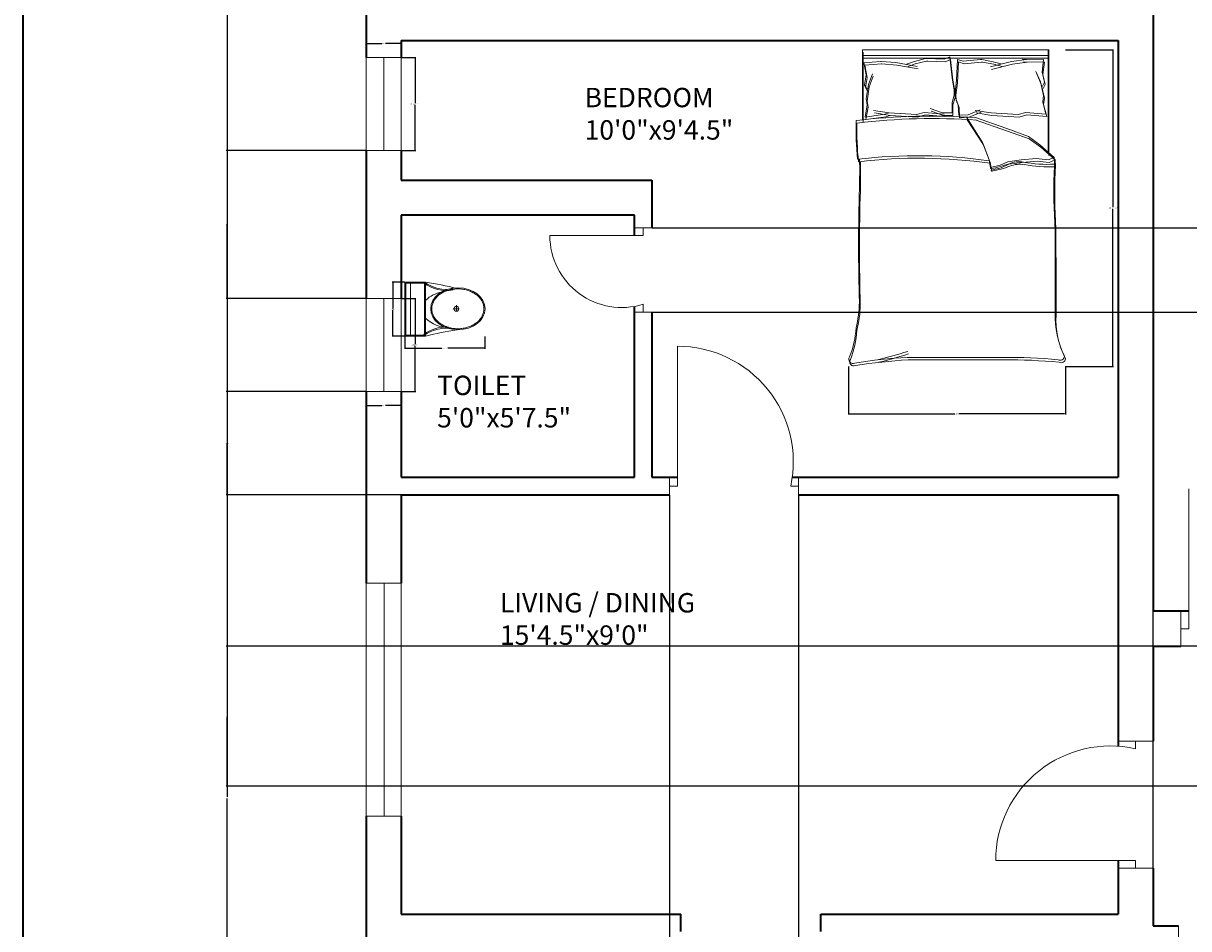
# Model space of a CAD drawing. Units: inches. Extents: x 2527 to 3140, y 1564 to 2435.
# Tile 2 of 4: x 2527 to 2827, y 1993 to 2227. Entities that reach past the tile are written whole.
import ezdxf

# ---------------------------------------------------------------- set-up
doc = ezdxf.new("R2010")
doc.units = ezdxf.units.IN
for name, color, linetype, lineweight in [('A-ANNO-DIMS', 2, 'Continuous', 18), ('A-ANNO-TTLB', 7, 'Continuous', 35), ('A-AREA-IDEN', 7, 'Continuous', 18), ('A-DOOR', 191, 'Continuous', 18), ('A-FLOR-FIXT', 7, 'Continuous', 18), ('A-FURN', 8, 'Continuous', 13), ('A-GLAZ', 131, 'Continuous', 18), ('A-WALL', 7, 'Continuous', 35)]:
    doc.layers.add(name, color=color, linetype=linetype, lineweight=lineweight)
doc.styles.get("Standard").update_dxf_attribs({"font": 'arial.ttf'})
doc.dimstyles.get("Standard").update_dxf_attribs({"dimtxt": 0.18, "dimasz": 0.18, "dimexe": 0.18, "dimexo": 0.0625, "dimgap": 0.09, "dimtad": 0, "dimtih": 1, "dimtoh": 1, "dimdec": 4, "dimzin": 0, "dimdsep": 46, "dimtxsty": 'Standard', "dimcen": 0.09, "dimadec": 0, "dimazin": 0, "dimtfac": 1, "dimtdec": 4, "dimtofl": 0, "dimtmove": 0, "dimatfit": 3, "dimfxl": 1, "dimtolj": 1, "dimtzin": 0, "dimarcsym": 0})

# ---------------------------------------------------------------- blocks, each defined once
blk = doc.blocks.new('A$C31115884')
for p, q in [((283, 498), (223, 498)), ((258, 466), (258, 523)), ((0, 200), (0, 0)), ((520, 200), (0, 200)), ((10, 190), (10, 10)), ((510, 190), (10, 190)), ((510, 10), (510, 190)), ((520, 0), (520, 200)), ((510, 54), (0, 54)), ((10, 10), (510, 10)), ((0, 0), (520, 0))]:
    blk.add_line(p, q)
blk.add_circle((256, 496), 23.6)
for centre, radius, start, end in [((2778, -205), 2807, 165.4549, 171.7133), ((-295, 403), 365, 324.2091, 9.3499), ((-295, 403), 375, 324.2091, 9.3499), ((806, 403), 365, 170.6501, 215.7909), ((3237, 905), 2807, 188.2867, 194.5451), ((384, 406), 293, 190.2774, 224.1564), ((139, 406), 293, 315.8436, 2.6563), ((806, 403), 375, 179.2036, 215.7909)]:
    blk.add_arc(centre, radius, start, end)
blk.add_ellipse((256, 510), major_axis=(0, -261), ratio=0.772727)
blk.add_open_spline([(256, 259), (263, 259), (270, 260), (288, 262), (299, 265), (320, 273), (330, 278), (350, 291), (360, 299), (378, 316), (386, 326), (402, 347), (409, 358), (421, 383), (427, 395), (436, 422), (440, 436), (445, 465), (447, 480), (448, 509), (448, 524), (445, 553), (443, 568), (436, 596), (432, 610), (422, 636), (416, 649), (402, 672), (395, 683), (379, 703), (370, 712), (351, 728), (341, 735), (321, 746), (310, 751), (289, 757), (278, 759), (256, 761), (245, 761), (223, 757), (212, 754), (191, 746), (181, 741), (161, 728), (151, 720), (133, 703), (125, 693), (110, 672), (103, 660), (90, 636), (85, 623), (76, 596), (72, 582), (67, 553), (66, 538), (64, 509), (65, 494), (68, 465), (70, 450), (77, 422), (81, 408), (91, 382), (97, 370), (111, 346), (118, 335), (135, 316), (144, 307), (162, 291), (172, 284), (193, 273), (203, 269), (225, 262), (236, 260), (250, 259), (253, 259), (256, 259)], degree=3, knots=[0, 0, 0, 0, 0.110105, 0.110105, 0.285049, 0.285049, 0.459994, 0.459994, 0.634938, 0.634938, 0.809882, 0.809882, 0.984827, 0.984827, 1.159771, 1.159771, 1.334715, 1.334715, 1.50966, 1.50966, 1.684604, 1.684604, 1.859549, 1.859549, 2.034493, 2.034493, 2.209437, 2.209437, 2.384382, 2.384382, 2.559326, 2.559326, 2.73427, 2.73427, 2.909215, 2.909215, 3.084159, 3.084159, 3.259103, 3.259103, 3.434048, 3.434048, 3.608992, 3.608992, 3.783936, 3.783936, 3.958881, 3.958881, 4.133825, 4.133825, 4.30877, 4.30877, 4.483714, 4.483714, 4.658658, 4.658658, 4.833603, 4.833603, 5.008547, 5.008547, 5.183491, 5.183491, 5.358436, 5.358436, 5.53338, 5.53338, 5.708324, 5.708324, 5.883269, 5.883269, 6.058213, 6.058213, 6.233158, 6.233158, 6.283185, 6.283185, 6.283185, 6.283185])
blk = doc.blocks.new('BED-DOUBLE')
for p, q in [((3.48, 63.33), (3.48, 81.44)), ((3.48, 63.33), (3.48, 81.44)), ((3.48, 81.44), (51.49, 81.44)), ((51.27, 81.44), (51.27, 54.83)), ((51.27, 81.44), (51.27, 54.83)), ((51.49, 81.44), (51.49, 80.8)), ((3.48, 79.91), (51.27, 79.91)), ((3.48, 79.91), (51.27, 79.91)), ((3.7, 62.69), (3.7, 80.8)), ((3.7, 62.69), (3.7, 80.8)), ((3.7, 79.27), (51.49, 79.27)), ((3.7, 79.27), (51.49, 79.27)), ((3.89, 78.13), (4.47, 74.95)), ((3.9, 78.1), (8.18, 78.43)), ((3.9, 78.1), (8.18, 78.43)), ((3.9, 78.13), (4.47, 74.95)), ((8.18, 78.43), (8.29, 78.42)), ((8.18, 78.43), (8.29, 78.42)), ((8.29, 78.42), (12.11, 78.13)), ((8.29, 78.42), (12.11, 78.13)), ((12.11, 78.13), (17.6, 77.11)), ((12.11, 78.13), (17.6, 77.11)), ((14.86, 77.69), (16.88, 78.42)), ((14.86, 77.69), (16.88, 78.42)), ((16.88, 78.42), (19.77, 79.14)), ((16.88, 78.42), (19.77, 79.14)), ((17.11, 77.78), (20, 78.5)), ((17.11, 77.78), (20, 78.5)), ((19.77, 79.14), (20.09, 79.14)), ((19.77, 79.14), (20.09, 79.14)), ((20, 78.5), (20.32, 78.5)), ((20, 78.5), (20.32, 78.5)), ((20.09, 79.14), (24.54, 78.99)), ((20.09, 79.14), (24.54, 78.99)), ((20.32, 78.5), (24.77, 78.35)), ((20.32, 78.5), (24.77, 78.35)), ((24.54, 78.99), (25.98, 79.57)), ((24.54, 78.99), (25.98, 79.57)), ((24.77, 78.35), (26.21, 78.93)), ((24.77, 78.35), (26.21, 78.93)), ((25.98, 79.57), (26.56, 74.22)), ((25.98, 79.57), (26.56, 74.22)), ((26.21, 78.93), (26.79, 73.58)), ((26.21, 78.93), (26.79, 73.58)), ((27.98, 78.95), (27.73, 73.58)), ((27.98, 78.95), (27.73, 73.58)), ((28.21, 78.31), (27.96, 72.94)), ((28.21, 78.31), (27.96, 72.94)), ((29.46, 78.46), (27.98, 78.95)), ((29.46, 78.46), (27.98, 78.95)), ((29.68, 77.82), (28.21, 78.31)), ((29.68, 77.82), (28.21, 78.31)), ((33.88, 78.89), (29.46, 78.46)), ((33.88, 78.89), (29.46, 78.46)), ((34.11, 78.25), (29.68, 77.82)), ((34.11, 78.25), (29.68, 77.82)), ((34.21, 78.91), (33.88, 78.89)), ((34.2, 78.91), (33.88, 78.89)), ((34.43, 78.27), (34.11, 78.25)), ((34.43, 78.27), (34.11, 78.25)), ((37.14, 78.36), (34.2, 78.91)), ((37.14, 78.36), (34.21, 78.91)), ((37.36, 77.73), (34.43, 78.27)), ((37.36, 77.73), (34.43, 78.27)), ((41.91, 78.37), (36.5, 77.02)), ((41.91, 78.37), (36.5, 77.02)), ((39.2, 77.77), (37.14, 78.36)), ((39.2, 77.77), (37.14, 78.36)), ((45.71, 78.9), (41.91, 78.37)), ((45.71, 78.9), (41.91, 78.37)), ((45.94, 78.26), (42.14, 77.73)), ((45.94, 78.26), (42.14, 77.73)), ((50.11, 78.89), (44.71, 78.98)), ((44.71, 78.98), (45.71, 78.9)), ((50.11, 78.89), (44.71, 78.98)), ((44.71, 78.98), (45.71, 78.9)), ((50.34, 78.25), (44.94, 78.34)), ((44.94, 78.34), (45.94, 78.26)), ((50.34, 78.25), (44.94, 78.34)), ((44.94, 78.34), (45.94, 78.26)), ((50.11, 78.89), (49.73, 75.68)), ((50.11, 78.89), (49.73, 75.68)), ((50.34, 78.25), (49.96, 75.04)), ((50.34, 78.25), (49.96, 75.04)), ((51.49, 80.8), (51.49, 54.19)), ((51.49, 80.8), (51.49, 54.19)), ((4.12, 77.49), (4.7, 74.31)), ((4.12, 77.49), (4.7, 74.31)), ((4.13, 77.47), (8.41, 77.79)), ((4.13, 77.47), (8.41, 77.79)), ((5.05, 72.49), (6.06, 75.24)), ((5.05, 72.49), (6.06, 75.24)), ((8.41, 77.79), (8.51, 77.78)), ((8.41, 77.79), (8.51, 77.78)), ((8.51, 77.78), (12.34, 77.49)), ((8.51, 77.78), (12.34, 77.49)), ((12.34, 77.49), (17.83, 76.48)), ((12.34, 77.49), (17.83, 76.48)), ((15.08, 77.05), (17.11, 77.78)), ((15.08, 77.05), (17.11, 77.78)), ((42.14, 77.73), (36.72, 76.38)), ((42.14, 77.73), (36.72, 76.38)), ((39.43, 77.13), (37.36, 77.73)), ((39.43, 77.13), (37.36, 77.73)), ((49.31, 73.19), (48.13, 75.86)), ((49.31, 73.19), (48.13, 75.86)), ((49.54, 72.55), (48.36, 75.23)), ((49.54, 72.55), (48.36, 75.23)), ((49.73, 75.68), (50.33, 73.1)), ((49.73, 75.68), (50.33, 73.1)), ((49.96, 75.04), (50.56, 72.47)), ((49.96, 75.04), (50.56, 72.47)), ((4.47, 74.95), (4.04, 72.34)), ((4.47, 74.95), (4.04, 72.34)), ((4.04, 72.34), (4.62, 71.33)), ((4.04, 72.34), (4.62, 71.33)), ((4.7, 74.31), (4.27, 71.7)), ((4.7, 74.31), (4.27, 71.7)), ((4.47, 68.87), (5.05, 72.49)), ((4.47, 68.87), (5.05, 72.49)), ((5.28, 71.85), (6.29, 74.6)), ((5.28, 71.85), (6.29, 74.6)), ((26.56, 74.22), (27.14, 71.04)), ((26.56, 74.22), (27.14, 71.04)), ((26.79, 73.58), (27.37, 70.4)), ((26.79, 73.58), (27.37, 70.4)), ((27.73, 73.58), (27.36, 70.36)), ((27.73, 73.58), (27.36, 70.36)), ((27.96, 72.94), (27.58, 69.73)), ((27.96, 72.94), (27.58, 69.73)), ((50.11, 69.61), (49.31, 73.19)), ((50.11, 69.61), (49.31, 73.19)), ((50.34, 68.97), (49.54, 72.55)), ((50.34, 68.97), (49.54, 72.55)), ((50.33, 73.1), (49.81, 72.06)), ((50.33, 73.1), (49.82, 72.06)), ((50.56, 72.47), (50.04, 71.42)), ((50.56, 72.47), (50.04, 71.42)), ((4.27, 71.7), (4.85, 70.69)), ((4.27, 71.7), (4.85, 70.69)), ((4.7, 68.23), (5.28, 71.85)), ((4.7, 68.23), (5.28, 71.85)), ((27.14, 69.74), (26.56, 67.86)), ((27.14, 69.74), (26.56, 67.86)), ((27.37, 69.1), (26.79, 67.22)), ((27.37, 69.1), (26.79, 67.22)), ((27.14, 71.04), (27.14, 69.74)), ((27.14, 71.04), (27.14, 69.74)), ((27.36, 70.36), (27.44, 69.07)), ((27.36, 70.36), (27.44, 69.07)), ((27.37, 70.4), (27.37, 69.1)), ((27.37, 70.4), (27.37, 69.1)), ((27.44, 69.07), (28.13, 67.23)), ((27.44, 69.07), (28.13, 67.23)), ((27.58, 69.73), (27.66, 68.43)), ((27.58, 69.73), (27.66, 68.43)), ((49.92, 68.01), (50.11, 69.61)), ((49.92, 68.01), (50.11, 69.61)), ((4.18, 64.1), (4.76, 67.28)), ((4.18, 64.1), (4.76, 67.28)), ((4.41, 63.46), (4.99, 66.64)), ((4.41, 63.46), (4.99, 66.64)), ((4.76, 67.28), (4.47, 68.87)), ((4.76, 67.28), (4.47, 68.87)), ((4.99, 66.64), (4.7, 68.23)), ((4.99, 66.64), (4.7, 68.23)), ((24.1, 65.18), (20.96, 66.27)), ((24.1, 65.18), (20.96, 66.27)), ((26.56, 67.86), (26.56, 65.18)), ((26.56, 67.86), (26.56, 65.18)), ((26.79, 67.22), (26.79, 64.54)), ((26.79, 67.22), (26.79, 64.54)), ((27.66, 68.43), (28.36, 66.59)), ((27.66, 68.43), (28.36, 66.59)), ((28.13, 67.23), (28.3, 64.55)), ((28.13, 67.23), (28.3, 64.55)), ((28.36, 66.59), (28.53, 63.91)), ((28.36, 66.59), (28.53, 63.91)), ((50.7, 64.87), (49.92, 68.01)), ((50.7, 64.87), (49.92, 68.01)), ((50.15, 67.37), (50.34, 68.97)), ((50.15, 67.37), (50.34, 68.97)), ((50.93, 64.23), (50.15, 67.37)), ((50.93, 64.23), (50.15, 67.37)), ((9.28, 64.82), (4.18, 64.1)), ((9.28, 64.82), (4.18, 64.1)), ((9.51, 64.19), (4.41, 63.46)), ((9.51, 64.19), (4.41, 63.46)), ((6.38, 65.81), (10.41, 65.15)), ((6.38, 65.81), (10.41, 65.15)), ((6.61, 65.17), (10.64, 64.51)), ((6.61, 65.17), (10.64, 64.51)), ((10.41, 65.15), (9.28, 64.82)), ((10.41, 65.15), (9.28, 64.82)), ((10.64, 64.51), (9.51, 64.19)), ((10.64, 64.51), (9.51, 64.19)), ((10.41, 65.15), (17.42, 64.72)), ((10.41, 65.15), (17.42, 64.72)), ((10.64, 64.51), (17.65, 64.08)), ((10.64, 64.51), (17.65, 64.08)), ((17.42, 64.72), (19.38, 65.27)), ((17.42, 64.72), (19.38, 65.27)), ((17.65, 64.08), (19.61, 64.63)), ((17.65, 64.08), (19.61, 64.63)), ((19.38, 65.27), (24.52, 64.87)), ((19.38, 65.27), (24.52, 64.87)), ((19.61, 64.63), (24.74, 64.23)), ((19.61, 64.63), (24.74, 64.23)), ((24.33, 64.54), (21.19, 65.63)), ((24.33, 64.54), (21.19, 65.63)), ((26.56, 65.18), (24.1, 65.18)), ((26.56, 65.18), (24.1, 65.18)), ((26.79, 64.54), (24.33, 64.54)), ((26.79, 64.54), (24.33, 64.54)), ((28.3, 64.55), (30.75, 64.7)), ((28.3, 64.55), (30.75, 64.7)), ((28.53, 63.91), (30.98, 64.06)), ((28.53, 63.91), (30.98, 64.06)), ((30.26, 64.06), (34.45, 57.57)), ((30.26, 64.06), (34.45, 57.57)), ((30.49, 63.42), (34.68, 56.93)), ((30.49, 63.42), (34.68, 56.93)), ((30.75, 64.7), (33.82, 65.99)), ((30.75, 64.7), (33.82, 65.99)), ((30.98, 64.06), (34.05, 65.35)), ((30.98, 64.06), (34.05, 65.35)), ((40.64, 61.13), (32.31, 64.06)), ((40.64, 61.13), (32.31, 64.06)), ((40.87, 60.49), (32.53, 63.42)), ((40.87, 60.49), (32.54, 63.42)), ((32.56, 65.81), (36.6, 65.15)), ((32.56, 65.81), (36.6, 65.15)), ((32.79, 65.17), (36.83, 64.51)), ((32.79, 65.17), (36.82, 64.51)), ((36.6, 65.15), (43.61, 64.72)), ((36.6, 65.15), (43.61, 64.72)), ((36.82, 64.51), (43.83, 64.08)), ((36.83, 64.51), (43.84, 64.08)), ((43.61, 64.72), (45.57, 65.27)), ((43.61, 64.72), (45.57, 65.27)), ((43.83, 64.08), (45.8, 64.63)), ((43.84, 64.08), (45.8, 64.63)), ((45.57, 65.27), (50.7, 64.87)), ((45.57, 65.27), (50.7, 64.87)), ((45.8, 64.63), (50.93, 64.23)), ((45.8, 64.63), (50.93, 64.23)), ((46.22, 59.11), (40.64, 61.13)), ((46.22, 59.11), (40.64, 61.13)), ((46.45, 58.47), (40.87, 60.49)), ((46.45, 58.47), (40.87, 60.49)), ((34.45, 57.57), (36.15, 53.08)), ((34.45, 57.57), (36.15, 53.08)), ((49.16, 56.95), (46.22, 59.11)), ((49.16, 56.95), (46.22, 59.11)), ((49.39, 56.31), (46.45, 58.47)), ((49.39, 56.31), (46.45, 58.47)), ((34.68, 56.93), (36.38, 52.44)), ((34.68, 56.93), (36.38, 52.44)), ((52.87, 53.7), (49.16, 56.95)), ((52.87, 53.7), (49.16, 56.95)), ((53.1, 53.06), (49.39, 56.31)), ((53.1, 53.06), (49.39, 56.31)), ((36.15, 53.08), (36.46, 51.07)), ((36.15, 53.08), (36.46, 51.07)), ((36.38, 52.44), (36.69, 50.43)), ((36.38, 52.44), (36.69, 50.43)), ((36.46, 51.07), (38.94, 51.68)), ((36.46, 51.07), (38.94, 51.68)), ((36.69, 50.43), (39.17, 51.05)), ((36.69, 50.43), (39.17, 51.05)), ((38.94, 51.68), (40.95, 52.61)), ((38.94, 51.68), (40.95, 52.61)), ((39.17, 51.05), (41.18, 51.97)), ((39.17, 51.05), (41.18, 51.97)), ((40.95, 52.61), (44.36, 53.08)), ((40.95, 52.61), (44.36, 53.08)), ((41.18, 51.97), (44.59, 52.44)), ((41.18, 51.97), (44.59, 52.44)), ((44.36, 53.08), (48.23, 53.39)), ((44.36, 53.08), (48.23, 53.39)), ((44.59, 52.44), (48.46, 52.75)), ((44.59, 52.44), (48.46, 52.75)), ((48.23, 53.39), (51.33, 53.08)), ((48.23, 53.39), (51.33, 53.08)), ((48.46, 52.75), (51.56, 52.44)), ((48.46, 52.75), (51.56, 52.44)), ((51.33, 53.08), (52.87, 53.7)), ((51.33, 53.08), (52.87, 53.7)), ((51.56, 52.44), (53.1, 53.06)), ((51.56, 52.44), (53.1, 53.06)), ((52.95, 51.95), (52.87, 53.7, 3.87)), ((52.95, 51.95), (52.87, 53.7, 3.87)), ((53.18, 51.31), (53.1, 53.06, 3.87)), ((53.18, 51.31), (53.1, 53.06, 3.87)), ((15.06, 2.2), (39.68, 2.2)), ((15.06, 2.2), (39.68, 2.2)), ((15.29, 1.56), (39.91, 1.56)), ((15.29, 1.56), (39.91, 1.56))]:
    blk.add_line(p, q)
for centre, radius, start, end in [((85.16, 61.35), 83.31, 178.7218, 185.604), ((85.16, 61.35), 83.31, 178.7218, 185.604), ((21.36, -100.61), 164.97, 86.0865, 96.7821), ((21.36, -100.61), 164.97, 86.0865, 96.7821), ((21.59, -101.25), 164.97, 86.0865, 96.7821), ((21.59, -101.25), 164.97, 86.0865, 96.7821), ((85.39, 60.71), 83.31, 178.7218, 185.604), ((85.39, 60.71), 83.31, 178.7218, 185.604), ((17.76, -74.87), 129.02, 81.7845, 96.9006), ((17.76, -74.87), 129.02, 81.7845, 96.9006), ((17.98, -75.51), 129.02, 81.7845, 96.9006), ((17.98, -75.51), 129.02, 81.7845, 96.9006), ((-167.31, 50.27), 170.11, 358.4762, 1.0082), ((-167.31, 50.27), 170.11, 358.4762, 1.0082), ((-167.08, 49.63), 170.11, 358.4762, 1.0082), ((-167.08, 49.63), 170.11, 358.4762, 1.0082), ((36.64, 51), 0.185, 160.2464, 271.1377), ((36.64, 51), 0.185, 160.2464, 271.1377), ((31.15, 79.96), 29.65, 280.6617, 289.8806), ((31.15, 79.96), 29.65, 280.6617, 289.8806), ((31.38, 79.32), 29.65, 280.6617, 289.8806), ((31.38, 79.32), 29.65, 280.6617, 289.8806), ((43.74, 46.38), 6.22, 78.6608, 113.7384), ((43.74, 46.38), 6.22, 78.6608, 113.7384), ((43.97, 45.74), 6.22, 78.6608, 113.7384), ((43.97, 45.74), 6.22, 78.6608, 113.7384), ((51.33, 88.1), 36.18, 259.8763, 272.5657), ((51.33, 88.1), 36.18, 259.8763, 272.5657), ((51.56, 87.46), 36.18, 259.8763, 272.5657), ((51.56, 87.46), 36.18, 259.8763, 272.5657), ((182.27, 45.13), 129.5, 176.9791, 183.8365), ((182.27, 45.13), 129.5, 176.9791, 183.8365), ((182.49, 44.49), 129.5, 176.9791, 183.8365), ((182.49, 44.49), 129.5, 176.9791, 183.8365), ((36.87, 50.36), 0.185, 160.2464, 271.1377), ((36.86, 50.36), 0.185, 160.2464, 271.1377), ((484.82, 30.83), 482.31, 178.2277, 181.7185), ((484.82, 30.83), 482.31, 178.2277, 181.7185), ((485.05, 30.19), 482.31, 178.2277, 181.7185), ((485.05, 30.19), 482.31, 178.2277, 181.7185), ((-4508.74, 13.62), 4561.86, 0.00217, 0.28689), ((-4508.74, 13.62), 4561.86, 0.00217, 0.28689), ((-4508.51, 12.98), 4561.86, 0.00217, 0.28689), ((-4508.51, 12.98), 4561.86, 0.00217, 0.28689), ((-26.9, 16.93), 29.63, 346.0648, 358.9113), ((-26.9, 16.93), 29.63, 346.0648, 358.9113), ((-26.67, 16.29), 29.63, 346.0648, 358.9113), ((-26.67, 16.29), 29.63, 346.0648, 358.9113), ((76.16, 12.78), 23.07, 177.4714, 206.4681), ((76.16, 12.78), 23.07, 177.4714, 206.4681), ((76.39, 12.14), 23.07, 177.4714, 206.4681), ((76.39, 12.14), 23.07, 177.4714, 206.4681), ((-21.66, 11.17), 23.56, 337.9751, 356.652), ((-21.66, 11.17), 23.56, 337.9751, 356.652), ((-21.43, 10.53), 23.56, 337.9751, 356.652), ((-21.43, 10.53), 23.56, 337.9751, 356.652), ((-17.22, 105.15), 106.46, 283.3832, 287.7053), ((-17.22, 105.15), 106.46, 283.3832, 287.7053), ((-16.99, 104.52), 106.46, 283.3832, 287.7053), ((-16.99, 104.52), 106.46, 283.3832, 287.7053), ((1.09, 1.73), 1.09, 146.1736, 293.4781), ((1.09, 1.73), 1.09, 146.1736, 293.4781), ((1.32, 1.09), 1.09, 146.1736, 293.4781), ((1.32, 1.09), 1.09, 146.1736, 293.4781), ((21.43, -119.39), 121.76, 92.9958, 99.4091), ((21.43, -119.39), 121.76, 92.9958, 99.4091), ((21.66, -120.03), 121.76, 92.9958, 99.4091), ((21.66, -120.03), 121.76, 92.9958, 99.4091), ((41.15, -130.83), 133.04, 84.4998, 90.6351), ((41.15, -130.83), 133.04, 84.4998, 90.6351), ((41.38, -131.47), 133.04, 84.4998, 90.6351), ((41.38, -131.47), 133.04, 84.4998, 90.6351), ((54.41, 2.57), 1.1, 242.6588, 356.02), ((54.41, 2.57), 1.1, 242.6588, 356.02), ((54.64, 1.93), 1.1, 242.6588, 356.02), ((54.64, 1.93), 1.1, 242.6588, 356.02)]:
    blk.add_arc(centre, radius, start, end)
blk = doc.blocks.new('WIN-24')
for p, q in [((4.5, 24), (0, 24)), ((0, 24), (9, 24)), ((0, 24), (0, 0)), ((4.5, 0), (4.5, 24)), ((9, 24), (9, 0)), ((0, 0), (9, 0)), ((9, 0), (4.5, 0))]:
    blk.add_line(p, q)
blk = doc.blocks.new('WIN-24-ALT')
for p, q in [((0, 0), (0, 9)), ((0, 9), (0, 4.5)), ((24, 9), (0, 9)), ((24, 4.5), (24, 9)), ((24, 9), (24, 0)), ((0, 4.5), (24, 4.5)), ((0, 0), (24, 0))]:
    blk.add_line(p, q)
blk = doc.blocks.new('*D9')
at = {"layer": 'A-ANNO-DIMS', "color": 0, "lineweight": -2, "transparency": 16777216}
for p, q in [((2795.58, 2219.76), (2807.93, 2219.76)), ((2807.75, 2219.58), (2807.75, 2179.17)), ((2807.75, 2138.39), (2807.75, 2178.8)), ((2795.58, 2138.21), (2807.93, 2138.21))]:
    blk.add_line(p, q, dxfattribs=at)
at = {"layer": 'A-ANNO-DIMS', "color": 0, "transparency": 16777216}
for points in [[(2807.72, 2219.58), (2807.78, 2219.58), (2807.75, 2219.76)], [(2807.72, 2138.39), (2807.78, 2138.39), (2807.75, 2138.21)]]:
    blk.add_solid(points, dxfattribs=at)
at = {"layer": 'Defpoints', "color": 0, "transparency": 16777216}
for p in [(2795.51, 2219.76), (2807.75, 2219.76), (2795.51, 2138.21)]:
    blk.add_point(p, dxfattribs=at)
at = {"layer": 'A-ANNO-DIMS', "color": 0, "transparency": 16777216, "insert": (2807.75, 2178.98), "char_height": 0.18, "attachment_point": 5}
blk.add_mtext('\\A1;DOUBLE BED 82 TYP.', dxfattribs=at)
blk = doc.blocks.new('*D10')
at = {"layer": 'A-ANNO-DIMS', "color": 0, "lineweight": -2, "transparency": 16777216}
for p, q in [((2739.69, 2138.15), (2739.69, 2125.8)), ((2795.51, 2138.15), (2795.51, 2125.8)), ((2739.87, 2125.98), (2767.07, 2125.98)), ((2795.33, 2125.98), (2768.13, 2125.98))]:
    blk.add_line(p, q, dxfattribs=at)
at = {"layer": 'A-ANNO-DIMS', "color": 0, "transparency": 16777216}
for points in [[(2739.87, 2126.01), (2739.87, 2125.95), (2739.69, 2125.98)], [(2795.33, 2126.01), (2795.33, 2125.95), (2795.51, 2125.98)]]:
    blk.add_solid(points, dxfattribs=at)
at = {"layer": 'Defpoints', "color": 0, "transparency": 16777216}
for p in [(2739.69, 2138.21), (2795.51, 2138.21), (2795.51, 2125.98)]:
    blk.add_point(p, dxfattribs=at)
at = {"layer": 'A-ANNO-DIMS', "color": 0, "transparency": 16777216, "insert": (2767.6, 2125.98), "char_height": 0.18, "attachment_point": 5}
blk.add_mtext('\\A1;56 TYP.', dxfattribs=at)
blk = doc.blocks.new('*D11')
at = {"layer": 'A-ANNO-DIMS', "color": 0, "lineweight": -2, "transparency": 16777216}
for p, q in [((2625.48, 2145.91), (2625.48, 2142.69)), ((2646.13, 2145.91), (2646.13, 2142.69)), ((2625.66, 2142.87), (2635.03, 2142.87)), ((2645.95, 2142.87), (2636.58, 2142.87))]:
    blk.add_line(p, q, dxfattribs=at)
at = {"layer": 'A-ANNO-DIMS', "color": 0, "transparency": 16777216}
for points in [[(2625.66, 2142.9), (2625.66, 2142.84), (2625.48, 2142.87)], [(2645.95, 2142.9), (2645.95, 2142.84), (2646.13, 2142.87)]]:
    blk.add_solid(points, dxfattribs=at)
at = {"layer": 'Defpoints', "color": 0, "transparency": 16777216}
for p in [(2625.48, 2145.97), (2646.13, 2145.97), (2646.13, 2142.87)]:
    blk.add_point(p, dxfattribs=at)
at = {"layer": 'A-ANNO-DIMS', "color": 0, "transparency": 16777216, "insert": (2635.81, 2142.87), "char_height": 0.18, "attachment_point": 5}
blk.add_mtext('\\A1;WC 21 TYP.', dxfattribs=at)
blk = doc.blocks.new('*D12')
at = {"layer": 'A-ANNO-DIMS', "color": 0, "lineweight": -2, "transparency": 16777216}
for p, q in [((2625.42, 2159.91), (2622.2, 2159.91)), ((2622.38, 2159.73), (2622.38, 2153.12)), ((2622.38, 2146.15), (2622.38, 2152.76)), ((2625.42, 2145.97), (2622.2, 2145.97))]:
    blk.add_line(p, q, dxfattribs=at)
at = {"layer": 'A-ANNO-DIMS', "color": 0, "transparency": 16777216}
for points in [[(2622.35, 2159.73), (2622.41, 2159.73), (2622.38, 2159.91)], [(2622.35, 2146.15), (2622.41, 2146.15), (2622.38, 2145.97)]]:
    blk.add_solid(points, dxfattribs=at)
at = {"layer": 'Defpoints', "color": 0, "transparency": 16777216}
for p in [(2625.48, 2159.91), (2622.38, 2145.97), (2625.48, 2145.97)]:
    blk.add_point(p, dxfattribs=at)
at = {"layer": 'A-ANNO-DIMS', "color": 0, "transparency": 16777216, "insert": (2622.38, 2152.94), "char_height": 0.18, "attachment_point": 5}
blk.add_mtext('\\A1;14 TYP.', dxfattribs=at)
blk = doc.blocks.new('*D13')
at = {"layer": 'A-ANNO-DIMS', "color": 0, "lineweight": -2, "transparency": 16777216}
for p, q in [((2624.64, 2155.71), (2628.36, 2155.71)), ((2628.18, 2155.53), (2628.18, 2143.89)), ((2628.18, 2131.89), (2628.18, 2143.52)), ((2624.64, 2131.71), (2628.36, 2131.71))]:
    blk.add_line(p, q, dxfattribs=at)
at = {"layer": 'A-ANNO-DIMS', "color": 0, "transparency": 16777216}
for points in [[(2628.15, 2155.53), (2628.21, 2155.53), (2628.18, 2155.71)], [(2628.15, 2131.89), (2628.21, 2131.89), (2628.18, 2131.71)]]:
    blk.add_solid(points, dxfattribs=at)
at = {"layer": 'Defpoints', "color": 0, "transparency": 16777216}
for p in [(2624.58, 2155.71), (2628.18, 2155.71), (2624.58, 2131.71)]:
    blk.add_point(p, dxfattribs=at)
at = {"layer": 'A-ANNO-DIMS', "color": 0, "transparency": 16777216, "insert": (2628.18, 2143.71), "char_height": 0.18, "attachment_point": 5}
blk.add_mtext('\\A1;WINDOW 24 TYP.', dxfattribs=at)
blk = doc.blocks.new('*D14')
at = {"layer": 'A-ANNO-DIMS', "color": 0, "lineweight": -2, "transparency": 16777216}
for p, q in [((2615.58, 2131.64), (2615.58, 2127.93)), ((2624.58, 2131.64), (2624.58, 2127.93)), ((2615.76, 2128.11), (2619.62, 2128.11)), ((2624.4, 2128.11), (2620.54, 2128.11))]:
    blk.add_line(p, q, dxfattribs=at)
at = {"layer": 'A-ANNO-DIMS', "color": 0, "transparency": 16777216}
for points in [[(2615.76, 2128.14), (2615.76, 2128.08), (2615.58, 2128.11)], [(2624.4, 2128.14), (2624.4, 2128.08), (2624.58, 2128.11)]]:
    blk.add_solid(points, dxfattribs=at)
at = {"layer": 'Defpoints', "color": 0, "transparency": 16777216}
for p in [(2615.58, 2131.71), (2624.58, 2131.71), (2624.58, 2128.11)]:
    blk.add_point(p, dxfattribs=at)
at = {"layer": 'A-ANNO-DIMS', "color": 0, "transparency": 16777216, "insert": (2620.08, 2128.11), "char_height": 0.18, "attachment_point": 5}
blk.add_mtext('\\A1;9 TYP.', dxfattribs=at)
blk = doc.blocks.new('*D17')
at = {"layer": 'A-ANNO-DIMS', "color": 0, "lineweight": -2, "transparency": 16777216}
for p, q in [((2624.64, 2217.79), (2628.36, 2217.79)), ((2628.18, 2217.61), (2628.18, 2205.97)), ((2628.18, 2193.97), (2628.18, 2205.6)), ((2624.64, 2193.79), (2628.36, 2193.79))]:
    blk.add_line(p, q, dxfattribs=at)
at = {"layer": 'A-ANNO-DIMS', "color": 0, "transparency": 16777216}
for points in [[(2628.15, 2217.61), (2628.21, 2217.61), (2628.18, 2217.79)], [(2628.15, 2193.97), (2628.21, 2193.97), (2628.18, 2193.79)]]:
    blk.add_solid(points, dxfattribs=at)
at = {"layer": 'Defpoints', "color": 0, "transparency": 16777216}
for p in [(2624.58, 2217.79), (2628.18, 2217.79), (2624.58, 2193.79)]:
    blk.add_point(p, dxfattribs=at)
at = {"layer": 'A-ANNO-DIMS', "color": 0, "transparency": 16777216, "insert": (2628.18, 2205.79), "char_height": 0.18, "attachment_point": 5}
blk.add_mtext('\\A1;ALT. WINDOW 24 TYP.', dxfattribs=at)
blk = doc.blocks.new('*D18')
at = {"layer": 'A-ANNO-DIMS', "color": 0, "lineweight": -2, "transparency": 16777216}
for p, q in [((2615.58, 2217.85), (2615.58, 2221.57)), ((2615.76, 2221.39), (2619.62, 2221.39)), ((2624.4, 2221.39), (2620.54, 2221.39)), ((2624.58, 2217.85), (2624.58, 2221.57))]:
    blk.add_line(p, q, dxfattribs=at)
at = {"layer": 'A-ANNO-DIMS', "color": 0, "transparency": 16777216}
for points in [[(2615.76, 2221.42), (2615.76, 2221.36), (2615.58, 2221.39)], [(2624.4, 2221.42), (2624.4, 2221.36), (2624.58, 2221.39)]]:
    blk.add_solid(points, dxfattribs=at)
at = {"layer": 'Defpoints', "color": 0, "transparency": 16777216}
for p in [(2615.58, 2221.39), (2615.58, 2217.79), (2624.58, 2217.79)]:
    blk.add_point(p, dxfattribs=at)
at = {"layer": 'A-ANNO-DIMS', "color": 0, "transparency": 16777216, "insert": (2620.08, 2221.39), "char_height": 0.18, "attachment_point": 5}
blk.add_mtext('\\A1;9 TYP.', dxfattribs=at)
blk = doc.blocks.new('*D20')
at = {"layer": 'A-ANNO-DIMS', "color": 0, "lineweight": -2, "transparency": 16777216}
for p, q in [((2615.52, 2348.14), (2579.55, 2348.14)), ((2579.73, 2347.96), (2579.73, 2027.32)), ((2579.73, 1706.32), (2579.73, 2026.96)), ((2615.52, 1706.14), (2579.55, 1706.14))]:
    blk.add_line(p, q, dxfattribs=at)
at = {"layer": 'A-ANNO-DIMS', "color": 0, "transparency": 16777216}
for points in [[(2579.7, 2347.96), (2579.76, 2347.96), (2579.73, 2348.14)], [(2579.7, 1706.32), (2579.76, 1706.32), (2579.73, 1706.14)]]:
    blk.add_solid(points, dxfattribs=at)
at = {"layer": 'Defpoints', "color": 0, "transparency": 16777216}
for p in [(2579.73, 2348.14), (2615.58, 2348.14), (2615.58, 1706.14)]:
    blk.add_point(p, dxfattribs=at)
at = {"layer": 'A-ANNO-DIMS', "color": 0, "transparency": 16777216, "insert": (2579.73, 2027.14), "char_height": 0.18, "attachment_point": 5}
blk.add_mtext('\\A1;642', dxfattribs=at)
blk = doc.blocks.new('*D26')
at = {"layer": 'A-ANNO-DIMS', "color": 0, "lineweight": -2, "transparency": 16777216}
for p, q in [((2818.08, 1994.21), (2818.08, 2384.17)), ((2818.26, 2383.99), (2857.88, 2383.99)), ((2898.29, 2383.99), (2858.67, 2383.99)), ((2898.47, 1994.21), (2898.47, 2384.17))]:
    blk.add_line(p, q, dxfattribs=at)
at = {"layer": 'A-ANNO-DIMS', "color": 0, "transparency": 16777216}
for points in [[(2818.26, 2384.02), (2818.26, 2383.96), (2818.08, 2383.99)], [(2898.29, 2384.02), (2898.29, 2383.96), (2898.47, 2383.99)]]:
    blk.add_solid(points, dxfattribs=at)
at = {"layer": 'Defpoints', "color": 0, "transparency": 16777216}
for p in [(2898.47, 2383.99), (2818.08, 1994.14), (2898.47, 1994.14)]:
    blk.add_point(p, dxfattribs=at)
at = {"layer": 'A-ANNO-DIMS', "color": 0, "transparency": 16777216, "insert": (2858.27, 2383.99), "char_height": 0.18, "attachment_point": 5}
blk.add_mtext('\\A1;80.39', dxfattribs=at)
blk = doc.blocks.new('*D28')
at = {"layer": 'A-ANNO-DIMS', "color": 0, "lineweight": -2, "transparency": 16777216}
for p, q in [((2898.4, 2066.14), (2579.55, 2066.14)), ((2579.73, 2065.96), (2579.73, 2048.32)), ((2579.73, 2030.32), (2579.73, 2047.96)), ((2898.4, 2030.14), (2579.55, 2030.14))]:
    blk.add_line(p, q, dxfattribs=at)
at = {"layer": 'A-ANNO-DIMS', "color": 0, "transparency": 16777216}
for points in [[(2579.7, 2065.96), (2579.76, 2065.96), (2579.73, 2066.14)], [(2579.7, 2030.32), (2579.76, 2030.32), (2579.73, 2030.14)]]:
    blk.add_solid(points, dxfattribs=at)
at = {"layer": 'Defpoints', "color": 0, "transparency": 16777216}
for p in [(2579.73, 2066.14), (2898.47, 2066.14), (2898.47, 2030.14)]:
    blk.add_point(p, dxfattribs=at)
at = {"layer": 'A-ANNO-DIMS', "color": 0, "transparency": 16777216, "insert": (2579.73, 2048.14), "char_height": 0.18, "attachment_point": 5}
blk.add_mtext('\\A1;36', dxfattribs=at)
blk = doc.blocks.new('*D30')
at = {"layer": 'A-ANNO-DIMS', "color": 0, "lineweight": -2, "transparency": 16777216}
for p, q in [((2689.14, 2173.9), (3083.61, 2173.9)), ((3083.43, 2173.72), (3083.43, 2163.23)), ((3083.43, 2152.37), (3083.43, 2162.87)), ((2689.14, 2152.19), (3083.61, 2152.19))]:
    blk.add_line(p, q, dxfattribs=at)
at = {"layer": 'A-ANNO-DIMS', "color": 0, "transparency": 16777216}
for points in [[(3083.4, 2173.72), (3083.46, 2173.72), (3083.43, 2173.9)], [(3083.4, 2152.37), (3083.46, 2152.37), (3083.43, 2152.19)]]:
    blk.add_solid(points, dxfattribs=at)
at = {"layer": 'Defpoints', "color": 0, "transparency": 16777216}
for p in [(2689.08, 2173.9), (3083.43, 2173.9), (2689.08, 2152.19)]:
    blk.add_point(p, dxfattribs=at)
at = {"layer": 'A-ANNO-DIMS', "color": 0, "transparency": 16777216, "insert": (3083.43, 2163.05), "char_height": 0.18, "attachment_point": 5}
blk.add_mtext('\\A1;21.714', dxfattribs=at)
blk = doc.blocks.new('*D31')
at = {"layer": 'A-ANNO-DIMS', "color": 0, "lineweight": -2, "transparency": 16777216}
for p, q in [((2615.52, 2193.79), (2579.55, 2193.79)), ((2579.73, 2193.61), (2579.73, 2174.93)), ((2579.73, 2155.89), (2579.73, 2174.56)), ((2615.52, 2155.71), (2579.55, 2155.71))]:
    blk.add_line(p, q, dxfattribs=at)
at = {"layer": 'A-ANNO-DIMS', "color": 0, "transparency": 16777216}
for points in [[(2579.7, 2193.61), (2579.76, 2193.61), (2579.73, 2193.79)], [(2579.7, 2155.89), (2579.76, 2155.89), (2579.73, 2155.71)]]:
    blk.add_solid(points, dxfattribs=at)
at = {"layer": 'Defpoints', "color": 0, "transparency": 16777216}
for p in [(2579.73, 2193.79), (2615.58, 2193.79), (2615.58, 2155.71)]:
    blk.add_point(p, dxfattribs=at)
at = {"layer": 'A-ANNO-DIMS', "color": 0, "transparency": 16777216, "insert": (2579.73, 2174.75), "char_height": 0.18, "attachment_point": 5}
blk.add_mtext('\\A1;38.08', dxfattribs=at)
blk = doc.blocks.new('*D32')
at = {"layer": 'A-ANNO-DIMS', "color": 0, "lineweight": -2, "transparency": 16777216}
for p, q in [((2615.52, 2131.71), (2579.55, 2131.71)), ((2579.73, 2131.53), (2579.73, 2118.61)), ((2579.73, 2105.32), (2579.73, 2118.24)), ((2624.52, 2105.14), (2579.55, 2105.14))]:
    blk.add_line(p, q, dxfattribs=at)
at = {"layer": 'A-ANNO-DIMS', "color": 0, "transparency": 16777216}
for points in [[(2579.7, 2131.53), (2579.76, 2131.53), (2579.73, 2131.71)], [(2579.7, 2105.32), (2579.76, 2105.32), (2579.73, 2105.14)]]:
    blk.add_solid(points, dxfattribs=at)
at = {"layer": 'Defpoints', "color": 0, "transparency": 16777216}
for p in [(2579.73, 2131.71), (2615.58, 2131.71), (2624.58, 2105.14)]:
    blk.add_point(p, dxfattribs=at)
at = {"layer": 'A-ANNO-DIMS', "color": 0, "transparency": 16777216, "insert": (2579.73, 2118.42), "char_height": 0.18, "attachment_point": 5}
blk.add_mtext('\\A1;26.563', dxfattribs=at)
blk = doc.blocks.new('*D33')
at = {"layer": 'A-ANNO-DIMS', "color": 0, "lineweight": -2, "transparency": 16777216}
for p, q in [((2693.66, 2105.08), (2693.66, 1670.11)), ((2726.85, 2105.08), (2726.85, 1670.11)), ((2693.84, 1670.29), (2709.86, 1670.29)), ((2726.67, 1670.29), (2710.65, 1670.29))]:
    blk.add_line(p, q, dxfattribs=at)
at = {"layer": 'A-ANNO-DIMS', "color": 0, "transparency": 16777216}
for points in [[(2693.84, 1670.32), (2693.84, 1670.26), (2693.66, 1670.29)], [(2726.67, 1670.32), (2726.67, 1670.26), (2726.85, 1670.29)]]:
    blk.add_solid(points, dxfattribs=at)
at = {"layer": 'Defpoints', "color": 0, "transparency": 16777216}
for p in [(2693.66, 2105.14), (2726.85, 2105.14), (2726.85, 1670.29)]:
    blk.add_point(p, dxfattribs=at)
at = {"layer": 'A-ANNO-DIMS', "color": 0, "transparency": 16777216, "insert": (2710.25, 1670.29), "char_height": 0.18, "attachment_point": 5}
blk.add_mtext('\\A1;33.18', dxfattribs=at)

msp = doc.modelspace()

# ---------------------------------------------------------------- linework, layer by layer
at = {"layer": 'A-ANNO-TTLB'}
msp.add_lwpolyline([(2527.301, 2435.1781), (3140.3962, 2435.1781), (3140.3962, 1564.3652), (2527.301, 1564.3652)], close=True, dxfattribs=at)
at = {"layer": 'A-DOOR'}
for p, q in [((2686.8292, 2171.9043), (2662.8292, 2171.9043)), ((2684.5792, 2173.9043), (2689.0792, 2173.9043)), ((2689.0792, 2173.9043), (2686.8292, 2173.9043)), ((2686.8292, 2173.9043), (2686.8292, 2171.9043)), ((2686.8292, 2152.1906), (2686.8292, 2154.1906)), ((2684.5792, 2152.1906), (2689.0792, 2152.1906)), ((2689.0792, 2152.1906), (2686.8292, 2152.1906)), ((2695.6634, 2107.3926), (2695.6634, 2143.3926)), ((2693.6634, 2109.6426), (2693.6634, 2105.1426)), ((2726.845, 2109.6426), (2726.845, 2105.1426)), ((2693.6634, 2105.1426), (2693.6634, 2107.3926)), ((2693.6634, 2107.3926), (2695.6634, 2107.3926)), ((2726.845, 2107.3926), (2724.845, 2107.3926)), ((2726.845, 2105.1426), (2726.845, 2107.3926)), ((2827.2549, 2070.6426), (2827.2549, 2106.6426)), ((2825.2549, 2075.1426), (2825.2549, 2066.1426)), ((2825.2549, 2066.1426), (2825.2549, 2070.6426)), ((2825.2549, 2070.6426), (2827.2549, 2070.6426)), ((2809.0792, 2041.7228), (2818.0792, 2041.7228)), ((2818.0792, 2041.7228), (2813.5792, 2041.7228)), ((2813.5792, 2041.7228), (2813.5792, 2039.7228)), ((2813.5792, 2010.9413), (2777.5792, 2010.9413)), ((2813.5792, 2008.9413), (2813.5792, 2010.9413)), ((2809.0792, 2008.9413), (2818.0792, 2008.9413)), ((2818.0792, 2008.9413), (2813.5792, 2008.9413)), ((2824.6085, 1994.1426), (2824.6085, 1985.1426))]:
    msp.add_line(p, q, dxfattribs=at)
for centre, radius, start, end in [((2681.3662, 2171.9043), 18.537, 180, 287.140124), ((2695.6634, 2113.5653), 29.8273, 348.056441, 90), ((2807.0844, 2010.9413), 29.5052, 77.283626, 180)]:
    msp.add_arc(centre, radius, start, end, dxfattribs=at)
at = {"layer": 'A-GLAZ'}
for p, q in [((2615.5792, 2082.3928), (2624.5792, 2082.3928)), ((2615.5792, 2082.3928), (2615.5792, 2022.3928)), ((2624.5792, 2082.3928), (2620.2215, 2082.3928)), ((2620.2215, 2082.3928), (2620.2215, 2022.3928)), ((2624.5792, 2082.3928), (2624.5792, 2022.3928)), ((2620.2215, 2022.3928), (2615.5792, 2022.3928)), ((2615.5792, 2022.3928), (2624.5792, 2022.3928))]:
    msp.add_line(p, q, dxfattribs=at)
at = {"layer": 'A-WALL'}
for p, q in [((2615.5792, 2252.1722), (2615.5792, 2217.785)), ((2818.0792, 2231.1426), (2818.0792, 2075.1426)), ((2624.5792, 2222.1426), (2809.0792, 2222.1426)), ((2624.5792, 2222.1426), (2624.5792, 2217.785)), ((2809.0792, 2222.1426), (2809.0792, 2109.6426)), ((2615.5792, 2193.785), (2615.5792, 2155.7055)), ((2624.5792, 2193.785), (2624.5792, 2186.1426)), ((2624.5792, 2186.1426), (2684.5792, 2186.1426)), ((2684.5792, 2186.1426), (2689.0792, 2186.1426)), ((2689.0792, 2186.1426), (2689.0792, 2173.9043)), ((2684.5792, 2177.1426), (2624.5792, 2177.1426)), ((2624.5792, 2177.1426), (2624.5792, 2155.7055)), ((2684.5792, 2171.9043), (2684.5792, 2177.1426)), ((2684.5792, 2109.6426), (2684.5792, 2153.6479)), ((2689.0792, 2152.1906), (2689.0792, 2109.6426)), ((2615.5792, 2131.7055), (2615.5792, 2082.3928)), ((2624.5792, 2131.7055), (2624.5792, 2109.6426)), ((2624.5792, 2109.6426), (2684.5792, 2109.6426)), ((2624.5792, 2109.6426), (2684.5792, 2109.6426)), ((2689.0792, 2109.6426), (2695.6634, 2109.6426)), ((2725.2317, 2109.6426), (2809.0792, 2109.6426)), ((2624.5792, 2105.1426), (2693.6634, 2105.1426)), ((2624.5792, 2105.1426), (2624.5792, 2082.3928)), ((2624.5792, 2105.1426), (2624.5792, 2082.3928)), ((2726.845, 2105.1426), (2809.0792, 2105.1426)), ((2809.0792, 2105.1426), (2809.0792, 2040.379)), ((2827.2549, 2075.1426), (2818.0792, 2075.1426)), ((2818.0792, 2066.1426), (2825.2549, 2066.1426)), ((2818.0792, 2066.1426), (2818.0792, 2041.7228)), ((2615.5792, 2022.3928), (2615.5792, 1983.547)), ((2624.5792, 2022.3928), (2624.5792, 1997.1426)), ((2624.5792, 2022.3928), (2624.5792, 1997.1426)), ((2809.0792, 2010.9413), (2809.0792, 1997.1426)), ((2818.0792, 2008.9413), (2818.0792, 1994.1426)), ((2624.5792, 1997.1426), (2696.5792, 1997.1426)), ((2692.0792, 1997.1426), (2696.5792, 1997.1426)), ((2696.5792, 1992.6426), (2696.5792, 1997.1426)), ((2732.5792, 1992.6426), (2732.5792, 1997.1426)), ((2732.5792, 1997.1426), (2809.0792, 1997.1426)), ((2818.0792, 1994.1426), (2824.6085, 1994.1426))]:
    msp.add_line(p, q, dxfattribs=at)

# ---------------------------------------------------------------- block references
at = {"layer": 'A-FLOR-FIXT', "xscale": 0.0268011493576733, "yscale": 0.0268011493576733, "zscale": 0.0268011493576733, "rotation": 270}
msp.add_blockref('A$C31115884', (2625.4797, 2159.9076), dxfattribs=at)
at = {"layer": 'A-FURN'}
msp.add_blockref('BED-DOUBLE', (2739.7762, 2138.3141), dxfattribs=at)
at = {"layer": 'A-GLAZ', "rotation": 90.00000000000026}
msp.add_blockref('WIN-24-ALT', (2624.5787, 2193.7851), dxfattribs=at)
at = {"layer": 'A-GLAZ'}
msp.add_blockref('WIN-24', (2615.579, 2131.706), dxfattribs=at)

# ---------------------------------------------------------------- texts
at = {"layer": 'A-AREA-IDEN', "char_height": 5, "attachment_point": 1}
for s, width, insert in [('BEDROOM\\P10\'0"x9\'4.5"', 99.848707, (2671.7778, 2209.9397)), ('TOILET\\P5\'0"x5\'7.5"', 86.757287, (2633.8082, 2135.8124)), ('LIVING / DINING\\P15\'4.5"x9\'0"', 147.775953, (2649.9716, 2079.8302))]:
    msp.add_mtext_dynamic_manual_height_columns(s, width=width, gutter_width=12.5, heights=[0], dxfattribs=dict(at, insert=insert))

# ---------------------------------------------------------------- dimensions: what is measured, and where the dimension line sits
at = {"layer": 'A-ANNO-DIMS'}
for base, p1, p2, picture, middle in [((2898.4651, 2383.9926), (2818.0792, 1994.1426), (2898.4651, 1994.1426), '*D26', (2858.2722, 2383.9926)), ((2726.845, 1670.2926), (2693.6634, 2105.1426), (2726.845, 2105.1426), '*D33', (2710.2542, 1670.2926))]:
    dim = msp.add_linear_dim(base=base, p1=p1, p2=p2, dimstyle='Standard', override={"dimdec": 2, "dimlfac": 1, "dimrnd": 0, "dimzin": 0, "dimdsep": 46, "dimlunit": 2}, dxfattribs=at)
    dim.commit()
    dim.dimension.update_dxf_attribs({"geometry": picture, "text_midpoint": middle})
for base, p1, p2, override, picture, middle in [((2579.7292, 2348.1426), (2615.5792, 1706.1426), (2615.5792, 2348.1426), {"dimdec": 0, "dimlfac": 1, "dimrnd": 0, "dimzin": 0, "dimdsep": 46, "dimlunit": 2}, '*D20', (2579.7292, 2027.1426)), ((2579.7292, 2193.785), (2615.5792, 2155.7055), (2615.5792, 2193.785), {"dimdec": 2, "dimlfac": 1, "dimrnd": 0, "dimzin": 0, "dimdsep": 46, "dimlunit": 2}, '*D31', (2579.7292, 2174.7453)), ((3083.4292, 2173.9043), (2689.0792, 2152.1906), (2689.0792, 2173.9043), {"dimdec": 3, "dimlfac": 1, "dimrnd": 0, "dimzin": 0, "dimdsep": 46, "dimlunit": 2}, '*D30', (3083.4292, 2163.0474)), ((2579.7292, 2131.7055), (2624.5792, 2105.1426), (2615.5792, 2131.7055), {"dimdec": 3, "dimlfac": 1, "dimrnd": 0, "dimzin": 0, "dimdsep": 46, "dimlunit": 2}, '*D32', (2579.7292, 2118.424)), ((2579.7292, 2066.1426), (2898.4651, 2030.1426), (2898.4651, 2066.1426), {"dimdec": 0, "dimlfac": 1, "dimrnd": 0, "dimzin": 0, "dimdsep": 46, "dimlunit": 2}, '*D28', (2579.7292, 2048.1426))]:
    dim = msp.add_linear_dim(base=base, p1=p1, p2=p2, angle=90, dimstyle='Standard', override=override, dxfattribs=at)
    dim.commit()
    dim.dimension.update_dxf_attribs({"geometry": picture, "text_midpoint": middle})
for base, p1, p2, angle, text, picture, middle in [((2615.5792, 2221.385), (2624.5792, 2217.785), (2615.5792, 2217.785), 180, '<> TYP.', '*D18', (2620.0792, 2221.385)), ((2807.7471, 2219.757), (2795.5148, 2138.2083), (2795.5148, 2219.757), 90, 'DOUBLE BED <> TYP.', '*D9', (2807.7471, 2178.9827)), ((2628.1792, 2217.785), (2624.5792, 2193.785), (2624.5792, 2217.785), 90, 'ALT. WINDOW <> TYP.', '*D17', (2628.1792, 2205.785)), ((2622.3819, 2145.971), (2625.4797, 2159.9076), (2625.4797, 2145.971), 270, '<> TYP.', '*D12', (2622.3819, 2152.9393)), ((2628.1792, 2155.7055), (2624.5792, 2131.7055), (2624.5792, 2155.7055), 90, 'WINDOW <> TYP.', '*D13', (2628.1792, 2143.7055))]:
    dim = msp.add_linear_dim(base=base, p1=p1, p2=p2, angle=angle, text=text, dimstyle='Standard', override={"dimdec": 0, "dimlfac": 1, "dimrnd": 0, "dimzin": 0, "dimdsep": 46, "dimlunit": 2}, dxfattribs=at)
    dim.commit()
    dim.dimension.update_dxf_attribs({"geometry": picture, "text_midpoint": middle})
for base, p1, p2, text, picture, middle in [((2646.1319, 2142.8732), (2625.4797, 2145.971), (2646.1319, 2145.971), 'WC <> TYP.', '*D11', (2635.8058, 2142.8732)), ((2795.5148, 2125.9761), (2739.6902, 2138.2083), (2795.5148, 2138.2083), '<> TYP.', '*D10', (2767.6025, 2125.9761)), ((2624.5792, 2128.1055), (2615.5792, 2131.7055), (2624.5792, 2131.7055), '<> TYP.', '*D14', (2620.0792, 2128.1055))]:
    dim = msp.add_linear_dim(base=base, p1=p1, p2=p2, text=text, dimstyle='Standard', override={"dimdec": 0, "dimlfac": 1, "dimrnd": 0, "dimzin": 0, "dimdsep": 46, "dimlunit": 2}, dxfattribs=at)
    dim.commit()
    dim.dimension.update_dxf_attribs({"geometry": picture, "text_midpoint": middle})

doc.saveas('drawing.dxf')
